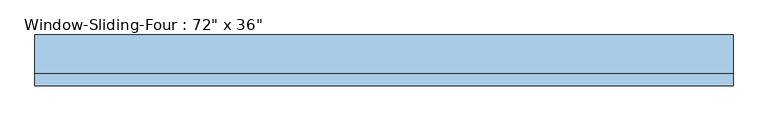
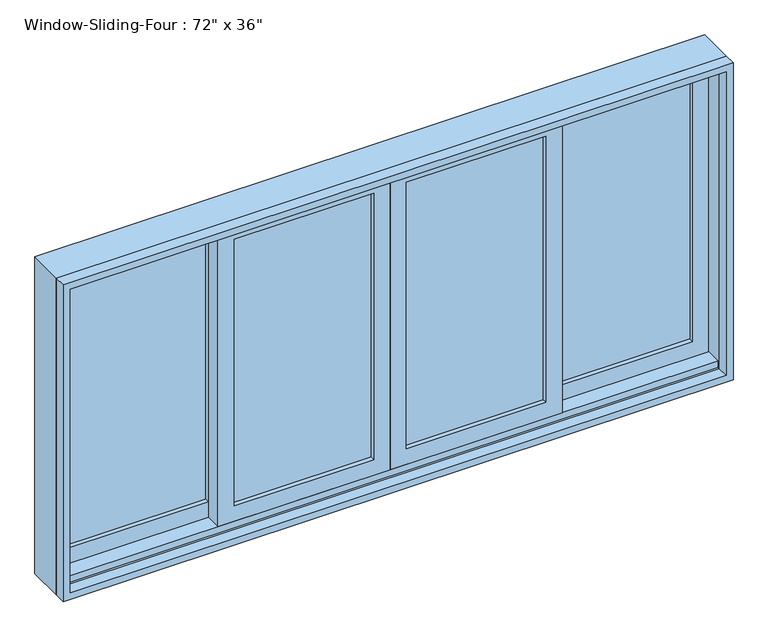
"""IFC4 building model written with IfcOpenShell, lengths in millimetres: window geometry."""

from ifc_helpers import new_model, si_unit, frame, origin, place, context, project, spatial, polyline, outline, extrude, faceted_brep, source, transform, mapped, element, save


def window_cd2bb1e7(model_context):
    return source(origin(), model_context, "Body", "SolidModel", [
        extrude(outline(polyline([(933.45, -895.35), (933.45, -425.45), (1809.75, -425.45), (1809.75, -895.35), (933.45, -895.35)]), holes=[polyline([(1765.3, -469.9), (996.95, -469.9), (996.95, -850.9), (1765.3, -850.9), (1765.3, -469.9)])]), frame((0.0, 21.59, 0.0), z_axis=(0.0, 1.0, 0.0), x_axis=(0.0, 0.0, 1.0)), (0.0, 0.0, 1.0), 44.45),
        extrude(outline(polyline([(-469.9, 53.34), (-469.9, 46.99), (-850.9, 46.99), (-850.9, 53.34), (-469.9, 53.34)])), frame((0.0, 0.0, 996.95), z_axis=(0.0, 0.0, 1.0), x_axis=(1.0, 0.0, 0.0)), (0.0, 0.0, 1.0), 768.35),
        extrude(outline(polyline([(-469.9, 40.64), (-469.9, 34.29), (-850.9, 34.29), (-850.9, 40.64), (-469.9, 40.64)])), frame((0.0, 0.0, 996.95), z_axis=(0.0, 0.0, 1.0), x_axis=(1.0, 0.0, 0.0)), (0.0, 0.0, 1.0), 768.35),
        extrude(outline(polyline([(-44.45, 8.89), (-44.45, 2.54), (-425.45, 2.54), (-425.45, 8.89), (-44.45, 8.89)])), frame((0.0, 0.0, 996.95), z_axis=(0.0, 0.0, 1.0), x_axis=(1.0, 0.0, 0.0)), (0.0, 0.0, 1.0), 768.35),
        extrude(outline(polyline([(-44.45, -3.81), (-44.45, -10.16), (-425.45, -10.16), (-425.45, -3.81), (-44.45, -3.81)])), frame((0.0, 0.0, 996.95), z_axis=(0.0, 0.0, 1.0), x_axis=(1.0, 0.0, 0.0)), (0.0, 0.0, 1.0), 768.35),
        extrude(outline(polyline([(1828.8, -914.4), (914.4, -914.4), (914.4, 914.4), (1828.8, 914.4), (1828.8, -914.4)]), holes=[polyline([(1809.75, 895.35), (933.45, 895.35), (933.45, -895.35), (1809.75, -895.35), (1809.75, 895.35)])]), frame((0.0, -60.96, 0.0), z_axis=(0.0, 1.0, 0.0), x_axis=(0.0, 0.0, 1.0)), (0.0, 0.0, 1.0), 31.75),
        extrude(outline(polyline([(952.5, 469.9), (1809.75, 469.9), (1809.75, 0.0), (952.5, 0.0), (952.5, 469.9)]), holes=[polyline([(996.95, 44.45), (1765.3, 44.45), (1765.3, 425.45), (996.95, 425.45), (996.95, 44.45)])]), frame((0.0, -22.86, 0.0), z_axis=(0.0, 1.0, 0.0), x_axis=(0.0, 0.0, 1.0)), (0.0, 0.0, 1.0), 44.45),
        extrude(outline(polyline([(1809.75, -469.9), (952.5, -469.9), (952.5, 0.0), (1809.75, 0.0), (1809.75, -469.9)]), holes=[polyline([(1765.3, -44.45), (996.95, -44.45), (996.95, -425.45), (1765.3, -425.45), (1765.3, -44.45)])]), frame((0.0, -22.86, 0.0), z_axis=(0.0, 1.0, 0.0), x_axis=(0.0, 0.0, 1.0)), (0.0, 0.0, 1.0), 44.45),
        extrude(outline(polyline([(425.45, 8.89), (425.45, 2.54), (44.45, 2.54), (44.45, 8.89), (425.45, 8.89)])), frame((0.0, 0.0, 996.95), z_axis=(0.0, 0.0, 1.0), x_axis=(1.0, 0.0, 0.0)), (0.0, 0.0, 1.0), 768.35),
        extrude(outline(polyline([(425.45, -3.81), (425.45, -10.16), (44.45, -10.16), (44.45, -3.81), (425.45, -3.81)])), frame((0.0, 0.0, 996.95), z_axis=(0.0, 0.0, 1.0), x_axis=(1.0, 0.0, 0.0)), (0.0, 0.0, 1.0), 768.35),
        extrude(outline(polyline([(850.9, 53.34), (850.9, 46.99), (469.9, 46.99), (469.9, 53.34), (850.9, 53.34)])), frame((0.0, 0.0, 996.95), z_axis=(0.0, 0.0, 1.0), x_axis=(1.0, 0.0, 0.0)), (0.0, 0.0, 1.0), 768.35),
        extrude(outline(polyline([(850.9, 40.3225303), (850.9, 34.29), (469.9, 34.29), (469.9, 40.3225303), (850.9, 40.3225303)])), frame((0.0, 0.0, 996.95), z_axis=(0.0, 0.0, 1.0), x_axis=(1.0, 0.0, 0.0)), (0.0, 0.0, 1.0), 768.35),
        extrude(outline(polyline([(933.45, 895.35), (1809.75, 895.35), (1809.75, 425.45), (933.45, 425.45), (933.45, 895.35)]), holes=[polyline([(1765.3, 469.9), (1765.3, 850.9), (996.95, 850.9), (996.95, 469.9), (1765.3, 469.9)])]), frame((0.0, 21.59, 0.0), z_axis=(0.0, 1.0, 0.0), x_axis=(0.0, 0.0, 1.0)), (0.0, 0.0, 1.0), 44.45),
        faceted_brep([(-914.4, -29.21, 914.4), (-914.4, 72.39, 914.4), (914.4, 72.39, 914.4), (914.4, -29.21, 914.4), (-873.4778905, 72.39, 1787.8778905), (-873.4778905, 66.04, 1787.8778905), (-873.4778905, 66.04, 933.45), (-873.4778905, 72.39, 933.45), (873.4778905, 66.04, 1787.8778905), (873.4778905, 66.04, 933.45), (895.35, 66.04, 933.45), (895.35, 66.04, 1809.75), (-895.35, 66.04, 1809.75), (-895.35, 66.04, 933.45), (-895.35, -29.21, 1809.75), (-895.35, -29.21, 933.45), (-895.35, -22.86, 933.45), (-895.35, -22.86, 952.5), (-895.35, 21.59, 952.5), (-895.35, 21.59, 933.45), (914.4, -29.21, 1828.8), (-914.4, -29.21, 1828.8), (895.35, -29.21, 1809.75), (895.35, -29.21, 933.45), (-914.4, 72.39, 1828.8), (914.4, 72.39, 1828.8), (873.4778905, 72.39, 933.45), (873.4778905, 72.39, 1787.8778905), (895.35, 21.59, 933.45), (895.35, 21.59, 952.5), (895.35, -22.86, 952.5), (895.35, -22.86, 933.45)], [[[0, 1, 2, 3]], [[4, 5, 6, 7]], [[5, 8, 9, 10, 11, 12, 13, 6]], [[12, 14, 15, 16, 17, 18, 19, 13]], [[0, 3, 20, 21], [22, 23, 15, 14]], [[24, 1, 0, 21]], [[2, 1, 24, 25], [4, 7, 26, 27]], [[5, 4, 27, 8]], [[12, 11, 22, 14]], [[21, 20, 25, 24]], [[8, 27, 26, 9]], [[22, 11, 10, 28, 29, 30, 31, 23]], [[20, 3, 2, 25]], [[26, 7, 6, 13, 19, 28, 10, 9]], [[28, 19, 18, 29]], [[29, 18, 17, 30]], [[30, 17, 16, 31]], [[15, 23, 31, 16]]]),
    ])


if __name__ == "__main__":
    model = new_model("IFC4")
    model_context = context("Model", 3, world=origin())
    ifc_project = project(units=[si_unit("LENGTHUNIT", "METRE", prefix="MILLI")], contexts=[model_context])
    site = spatial("IfcSite", under=ifc_project)
    building = spatial("IfcBuilding", under=site)
    placement = place(None, origin())
    window_shape = window_cd2bb1e7(model_context)
    element("IfcWindow", 1, ObjectType="Window-Sliding-Four : 72\" x 36\"", at=placement, inside=building, context=model_context, shape_type="MappedRepresentation", body=[
        mapped(window_shape, transform((0.0, 0.0, 0.0), x_axis=(1.0, 0.0, 0.0), y_axis=(0.0, 1.0, 0.0), z_axis=(0.0, 0.0, 1.0))),
    ])
    save(model, "model.ifc")

# Revit data of these elements
# Type "Window-Sliding-Four : 72\" x 36\""
#   Type Mark = "20"
#   Fire Rating = "0.5h"
#   Assembly Code = "B2020100"
#   Analytic Construction = "Double glazing - domestic"
#   Window Inset [instance default] = 0 ft
#   Wall Thickness [instance default] = 0.5 ft
#   Visual Light Transmittance = 0.81
#   Thermal Resistance (R) = 1.8146 (h·ft²·°F)/BTU
#   Solar Heat Gain Coefficient = 0.76
#   Interior Wall Closure [instance default] = 0.216146 ft
#   Heat Transfer Coefficient (U) = 0.5511 BTU/(h·ft²·°F)
#   Frame Extension [instance default] = 0.020833 ft
#   Exterior Wall Closure [instance default] = 0.104167 ft
#   Rough Width = 6.041667 ft
#   Rough Height = 3.041667 ft
#   Height = 3 ft
#   Extension Jamb [instance default] = 0.229167 ft
#   Default Sill Height = 3 ft
#   Width = 6 ft
#   Middle Muntin Visibility = yes
#   Interior Trim Visibility [instance default] = yes
#   Indicator Visibility [instance default] = yes
#   Exterior Trim Visibility [instance default] = yes
#   Side Muntin Visibility = yes
#   Extension Jamb Visibility [instance default] = yes
#   Interior Trim Material = Wood - Stained
#   Muntin Pattern = Muntin Pattern_2x2 : Muntin Pattern_2x2
#   Interior Trim = Trim-Window-Interior-Flat : Picture Frame
#   Interior Frame Material = Wood - Stained
#   Glass Panel Material = Glass
#   Exterior Trim Material = Clad - White
#   Exterior Trim = Trim-Window-Exterior-Flat : with Sill
#   Exterior Frame Material = Clad - White
#   Wall Closure = (empty or 0)
# Element 1 (IfcWindow, "Window-Sliding-Four : 72\" x 36\"")
#   Wall Thickness = 0.375 ft
#   Extension Jamb = 0.104167 ft
#   Materials on its faces: "Wood - Stained", "Glass", "Clad - White"
# Materials
#   "Wood - Stained": class "Wood", colour RGB 224 178 126, transparency 0, Cost = 0
#   "Glass": class "Glass", colour RGB 0 128 192, transparency 0.75, Description = "Soda Lime Glass", Cost = 0
#   "Clad - White": class "Wood", colour RGB 242 242 238, transparency 0, Cost = 0
